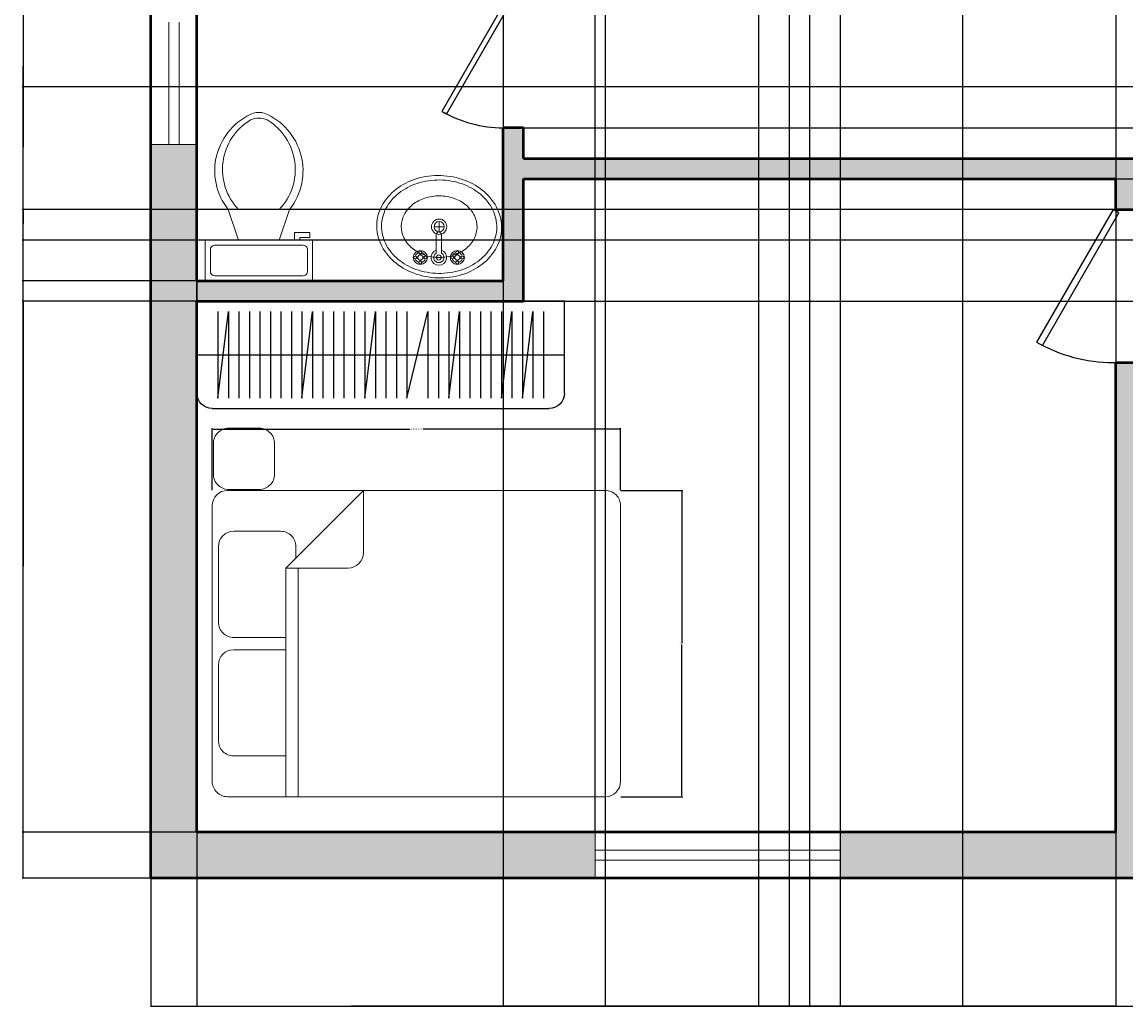
# Model space of a CAD drawing. Units: inches. Extents: x 3439 to 3988, y 1915 to 2284.
# Tile 1 of 7: x 3439 to 3656, y 1915 to 2108. Entities that reach past the tile are written whole.
import ezdxf

# ---------------------------------------------------------------- set-up
doc = ezdxf.new("R2010")
doc.units = ezdxf.units.IN
for name, color, linetype, lineweight in [('A-ANNO-DIMS', 2, 'Continuous', 18), ('A-DOOR', 3, 'Continuous', 25), ('A-FLOR-CASE', 8, 'Continuous', 25), ('A-FLOR-FIXT', 9, 'Continuous', 18), ('A-FURN', 9, 'Continuous', 18), ('A-GLAZ', 4, 'Continuous', 18), ('A-WALL', 7, 'Continuous', 50)]:
    doc.layers.add(name, color=color, linetype=linetype, lineweight=lineweight)
doc.layers.add('A-WALL-PATT', color=18, linetype='Continuous', lineweight=13, true_color=0x000000)
doc.styles.get("Standard").update_dxf_attribs({"font": 'arial.ttf'})
doc.dimstyles.get("Standard").update_dxf_attribs({"dimtxt": 0.18, "dimasz": 0.18, "dimexe": 0.18, "dimexo": 0.0625, "dimgap": 0.09, "dimtad": 0, "dimtih": 1, "dimtoh": 1, "dimdec": 4, "dimzin": 0, "dimdsep": 46, "dimtxsty": 'Standard', "dimcen": 0.09, "dimadec": 0, "dimazin": 0, "dimtfac": 1, "dimtdec": 4, "dimtofl": 0, "dimtmove": 0, "dimatfit": 3, "dimfxl": 1, "dimtolj": 1, "dimtzin": 0, "dimarcsym": 0})

# ---------------------------------------------------------------- blocks, each defined once
blk = doc.blocks.new('*U5')
for p, q in [((0, 0), (0, 6)), ((40, 0), (40, 6))]:
    blk.add_line(p, q)
blk.add_lwpolyline([(0, 0), (34.64, -20), (35.52, -18.48), (0.87, 1.52)], close=True)
blk.add_arc((0, 0), 40, 330, 0)
blk = doc.blocks.new('Bed - Queen')
for p, q in [((3, 0), (56.99999, 0)), ((10.99999, -1.2), (25.79998, -1.2)), ((34.19999, -1.2), (48.99999, -1.2)), ((0, -77.00003), (0, -3)), ((7.99999, -14.4), (7.99999, -4.2)), ((28.79998, -4.2), (28.79998, -14.4)), ((31.19999, -14.4), (31.19999, -4.2)), ((51.99999, -4.2), (51.99999, -13.4)), ((59.99999, -3), (59.99999, -77.00003)), ((0, -14.4), (44.8, -14.4)), ((59.99999, -29.6), (44.8, -14.4)), ((44.8, -14.4), (44.8, -26.6)), ((44.8, -16.8), (0, -16.8)), ((48.99999, -16.4), (46.79936, -16.4)), ((47.8, -29.6), (59.99999, -29.6)), ((56.99999, -80.00003), (3, -80.00003))]:
    blk.add_line(p, q)
for centre, start, end in [((3, -3), 90, 180), ((56.99999, -3), 0, 90), ((10.99999, -4.2), 90, 180), ((25.79998, -4.2), 0, 90), ((34.19999, -4.2), 90, 180), ((48.99999, -4.2), 0, 90), ((48.99999, -13.4), 270, 0), ((47.8, -26.6), 180, 270), ((3, -77.00003), 180, 270), ((56.99999, -77.00003), 270, 0)]:
    blk.add_arc(centre, 3, start, end)
blk = doc.blocks.new('Toilet - top')
for p, q in [((9.5, -6), (9.5, -2)), ((-10, -8.5), (-8, -8.5)), ((-10, -9.5), (-10, -8.5)), ((-8, -8.5), (-8, -8)), ((-7, -8), (-7, -9.5)), ((-4, -8), (-6, -14)), ((4, -8), (6, -14)), ((-7, -9.5), (-10, -9.5)), ((4, -14), (-4, -14))]:
    blk.add_line(p, q)
blk.add_lwpolyline([(10.5, -8), (10.5, 0), (-10.5, 0), (-10.5, -8)], close=True)
for points in [[(-9.5, -2), (-9.5, -6)], [(8.5, -1), (-8.5, -1)], [(-8.5, -7), (8.5, -7)]]:
    blk.add_lwpolyline(points)
for centre, radius, start, end in [((-8.62, -1.88), 0.884, 81.8699, 188.1301), ((8.62, -1.88), 0.884, 351.8699, 98.1301), ((-8.62, -6.12), 0.884, 171.8699, 278.1301), ((8.62, -6.12), 0.884, 261.8699, 8.1301), ((3.52, -21.58), 12.17, 141.4691, 247.9714), ((4.2, -21.82), 11.33, 136.3677, 238.9468), ((-3.52, -21.58), 12.17, 292.0284, 38.5307), ((-4.2, -21.82), 11.33, 301.053, 43.6321), ((0, -27.88), 4, 245.7318, 294.2682), ((0, -29), 4, 254.8605, 285.1395)]:
    blk.add_arc(centre, radius, start, end)
blk = doc.blocks.new('Sink - Oval top')
for p, q in [((-1, 0), (1, 0)), ((0, 1), (0, -1))]:
    blk.add_line(p, q)
for points in [[(-12.23, 0.39, 0.117634), (-11.46, -3.36, 0.104469), (-8.88, -6.8, 0.090016), (-5.08, -9.07, 0.08192), (-0.32, -10.02, 0.08192), (4.49, -9.38, 0.090016), (8.42, -7.36, 0.104469), (11.22, -4.09, 0.117634), (12.23, -0.39, 0.117634), (11.46, 3.36, 0.104469), (8.88, 6.8, 0.090016), (5.08, 9.07, 0.08192), (0.32, 10.02, 0.08192), (-4.49, 9.38, 0.090016), (-8.42, 7.36, 0.104469), (-11.22, 4.09, 0.117634)], [(-11.29, 0.16, 0.118622), (-10.52, -3.25, 0.104678), (-8.07, -6.36, 0.089562), (-4.54, -8.37, 0.081185), (-0.13, -9.15, 0.081185), (4.3, -8.49, 0.089562), (7.89, -6.58, 0.104678), (10.42, -3.55, 0.118622), (11.29, -0.16, 0.118622), (10.52, 3.25, 0.104678), (8.07, 6.36, 0.089562), (4.54, 8.37, 0.081185), (0.13, 9.15, 0.081185), (-4.3, 8.49, 0.089562), (-7.89, 6.58, 0.104678), (-10.42, 3.55, 0.118622)], [(-7.42, 0.08, 0.118283), (-6.91, -2.17, 0.104607), (-5.29, -4.21, 0.089718), (-2.97, -5.53, 0.081436), (-0.07, -6.04, 0.081436), (2.84, -5.59, 0.089718), (5.2, -4.33, 0.104607), (6.86, -2.32, 0.118283), (7.42, -0.08, 0.118283), (6.91, 2.17, 0.104607), (5.29, 4.21, 0.089718), (2.97, 5.53, 0.081436), (0.07, 6.04, 0.081436), (-2.84, 5.59, 0.089718), (-5.2, 4.33, 0.104607), (-6.86, 2.32, 0.118283)]]:
    blk.add_lwpolyline(points, format="xyb", close=True)
for radius in [1.5, 1]:
    blk.add_circle((0, 0), radius)
blk = doc.blocks.new('Faucet - Bathroom top')
for p, q in [((-4.107, 0.125), (-4.375, 0.125)), ((-3.75, 0.4788), (-3.75, 0.75)), ((-3.5, 0.482), (-3.5, 0.75)), ((-3.1461, 0.125), (-2.875, 0.125)), ((3.143, 0.125), (2.875, 0.125)), ((3.5, 0.4788), (3.5, 0.75)), ((3.75, 0.482), (3.75, 0.75)), ((4.1039, 0.125), (4.375, 0.125)), ((-4.1039, -0.125), (-4.375, -0.125)), ((-3.75, -0.4821), (-3.75, -0.75)), ((-3.5, -0.4789), (-3.5, -0.75)), ((-3.143, -0.125), (-2.875, -0.125)), ((-0.5, -0.8639), (-0.5, -4.5)), ((0.5, -4.5), (0.5, -0.8631)), ((3.1461, -0.125), (2.875, -0.125)), ((3.5, -0.4821), (3.5, -0.75)), ((3.75, -0.4789), (3.75, -0.75)), ((4.107, -0.125), (4.375, -0.125))]:
    blk.add_line(p, q)
for centre, radius in [((-3.625, 0), 1.375), ((-4.625, 0), 0.2795), ((-3.625, 0), 0.5), ((-3.625, 1), 0.2795), ((-2.625, 0), 0.2795), ((0, 0), 0.5), ((3.625, 0), 1.375), ((2.625, 0), 0.2795), ((3.625, 0), 0.5), ((3.625, 1), 0.2795), ((4.625, 0), 0.2795), ((-3.625, -1), 0.2795), ((3.625, -1), 0.2795)]:
    blk.add_circle(centre, radius)
for centre, radius, start, end in [((-3.625, 0), 1, 105.2407, 164.2093), ((-3.625, 0), 1, 16.44125, 74.07887), ((0, 0), 1.5, 289.6514, 250.3603), ((0, 0), 1, 300.3431, 239.7554), ((3.625, 0), 1, 106.12, 164.0884), ((3.625, 0), 1, 16.23422, 73.90469), ((-3.625, 0), 1, 196.2342, 253.9047), ((-3.625, 0), 1, 286.12, 344.0884), ((3.625, 0), 1, 196.4413, 254.0789), ((3.625, 0), 1, 285.2407, 344.2093), ((0, -4.5), 0.5, 180, 0)]:
    blk.add_arc(centre, radius, start, end)
blk = doc.blocks.new('WINDOW-GLASS-48IN')
for p, q in [((0, 2), (48, 2)), ((0, 0), (48, 0))]:
    blk.add_line(p, q)
blk = doc.blocks.new('WINDOW-GLASS-24IN')
for p, q in [((0, 2), (24, 2)), ((0, 0), (24, 0))]:
    blk.add_line(p, q)
blk = doc.blocks.new('WARDROBE-72IN')
for p, q in [((3, 21), (69, 21)), ((0, 0), (0, 18)), ((4.11, 2), (4.11, 19)), ((4.11, 19), (6.17, 2)), ((6.17, 2), (6.17, 19)), ((8.23, 2), (8.23, 19)), ((10.28, 2), (10.28, 19)), ((12.34, 2), (12.34, 19)), ((14.4, 2), (14.4, 19)), ((16.45, 2), (16.45, 19)), ((18.51, 2), (18.51, 19)), ((20.57, 2), (20.57, 19)), ((20.57, 19), (22.62, 2)), ((22.62, 2), (22.62, 19)), ((24.68, 2), (24.68, 19)), ((26.74, 2), (26.74, 19)), ((28.79, 2), (28.79, 19)), ((30.85, 2), (30.85, 19)), ((32.91, 2), (32.91, 19)), ((32.91, 19), (34.97, 2)), ((34.97, 2), (34.97, 19)), ((37.02, 2), (37.02, 19)), ((39.08, 2), (39.08, 19)), ((41.14, 2), (41.14, 19)), ((41.14, 19), (45.25, 2)), ((45.25, 2), (45.25, 19)), ((47.31, 2), (47.31, 19)), ((49.36, 2), (49.36, 19)), ((49.36, 19), (51.42, 2)), ((51.42, 2), (51.42, 19)), ((53.48, 2), (53.48, 19)), ((55.53, 2), (55.53, 19)), ((57.59, 2), (57.59, 19)), ((59.65, 2), (59.65, 19)), ((59.65, 19), (61.7, 2)), ((61.7, 2), (61.7, 19)), ((63.76, 2), (63.76, 19)), ((63.76, 19), (65.82, 2)), ((65.82, 2), (65.82, 19)), ((67.87, 2), (67.87, 19)), ((72, 18), (72, 0)), ((0, 10.5), (72, 10.5)), ((72, 0), (0, 0))]:
    blk.add_line(p, q)
for centre, start, end in [((3, 18), 90, 180), ((69, 18), 0, 90)]:
    blk.add_arc(centre, 3, start, end)
blk = doc.blocks.new('NIGHTSTAND-12IN-RADIUS')
blk.add_lwpolyline([(3, 0), (9, 0, 0.414214), (12, 3), (12, 9, 0.414214), (9, 12), (3, 12, 0.414214), (0, 9), (0, 3, 0.414214)], format="xyb", close=True)
blk = doc.blocks.new('*D23')
at = {"layer": 'A-ANNO-DIMS', "color": 0, "lineweight": -2, "transparency": 16777216}
for p, q in [((3476.58, 2016.37), (3476.58, 2028.49)), ((3556.58, 2016.37), (3556.58, 2028.49)), ((3476.76, 2028.31), (3515.28, 2028.31)), ((3556.4, 2028.31), (3517.89, 2028.31))]:
    blk.add_line(p, q, dxfattribs=at)
at = {"layer": 'A-ANNO-DIMS', "color": 0, "transparency": 16777216}
for points in [[(3476.76, 2028.34), (3476.76, 2028.28), (3476.58, 2028.31)], [(3556.4, 2028.34), (3556.4, 2028.28), (3556.58, 2028.31)]]:
    blk.add_solid(points, dxfattribs=at)
at = {"layer": 'Defpoints', "color": 0, "transparency": 16777216}
for p in [(3476.58, 2028.31), (3476.58, 2016.31), (3556.58, 2016.31)]:
    blk.add_point(p, dxfattribs=at)
at = {"layer": 'A-ANNO-DIMS', "color": 0, "transparency": 16777216, "insert": (3516.58, 2028.31), "char_height": 0.18, "attachment_point": 5}
blk.add_mtext('\\A1;QUEEN BED 80 TYP.', dxfattribs=at)
blk = doc.blocks.new('*D24')
at = {"layer": 'A-ANNO-DIMS', "color": 0, "lineweight": -2, "transparency": 16777216}
for p, q in [((3556.65, 2016.31), (3568.76, 2016.31)), ((3568.58, 2016.13), (3568.58, 1986.49)), ((3568.58, 1956.49), (3568.58, 1986.13)), ((3556.65, 1956.31), (3568.76, 1956.31))]:
    blk.add_line(p, q, dxfattribs=at)
at = {"layer": 'A-ANNO-DIMS', "color": 0, "transparency": 16777216}
for points in [[(3568.55, 2016.13), (3568.61, 2016.13), (3568.58, 2016.31)], [(3568.55, 1956.49), (3568.61, 1956.49), (3568.58, 1956.31)]]:
    blk.add_solid(points, dxfattribs=at)
at = {"layer": 'Defpoints', "color": 0, "transparency": 16777216}
for p in [(3556.58, 2016.31), (3568.58, 2016.31), (3556.58, 1956.31)]:
    blk.add_point(p, dxfattribs=at)
at = {"layer": 'A-ANNO-DIMS', "color": 0, "transparency": 16777216, "insert": (3568.58, 1986.31), "char_height": 0.18, "attachment_point": 5}
blk.add_mtext('\\A1;60 TYP.', dxfattribs=at)
blk = doc.blocks.new('*D45')
at = {"layer": 'A-ANNO-DIMS', "color": 0, "lineweight": -2, "transparency": 16777216}
for p, q in [((3464.58, 1940.3), (3464.58, 1915.13)), ((3962.58, 1940.3), (3962.58, 1915.13)), ((3464.76, 1915.31), (3713.29, 1915.31)), ((3962.4, 1915.31), (3713.87, 1915.31))]:
    blk.add_line(p, q, dxfattribs=at)
at = {"layer": 'A-ANNO-DIMS', "color": 0, "transparency": 16777216}
for points in [[(3464.76, 1915.34), (3464.76, 1915.28), (3464.58, 1915.31)], [(3962.4, 1915.34), (3962.4, 1915.28), (3962.58, 1915.31)]]:
    blk.add_solid(points, dxfattribs=at)
at = {"layer": 'Defpoints', "color": 0, "transparency": 16777216}
for p in [(3464.58, 1940.36), (3962.58, 1940.36), (3962.58, 1915.31)]:
    blk.add_point(p, dxfattribs=at)
at = {"layer": 'A-ANNO-DIMS', "color": 0, "transparency": 16777216, "insert": (3713.58, 1915.31), "char_height": 0.18, "attachment_point": 5}
blk.add_mtext('\\A1;498', dxfattribs=at)
blk = doc.blocks.new('*D46')
at = {"layer": 'A-ANNO-DIMS', "color": 0, "lineweight": -2, "transparency": 16777216}
for p, q in [((3464.52, 2258.36), (3439.35, 2258.36)), ((3439.53, 2258.18), (3439.53, 2099.54)), ((3439.53, 1940.54), (3439.53, 2099.18)), ((3464.52, 1940.36), (3439.35, 1940.36))]:
    blk.add_line(p, q, dxfattribs=at)
at = {"layer": 'A-ANNO-DIMS', "color": 0, "transparency": 16777216}
for points in [[(3439.5, 2258.18), (3439.56, 2258.18), (3439.53, 2258.36)], [(3439.5, 1940.54), (3439.56, 1940.54), (3439.53, 1940.36)]]:
    blk.add_solid(points, dxfattribs=at)
at = {"layer": 'Defpoints', "color": 0, "transparency": 16777216}
for p in [(3439.53, 2258.36), (3464.58, 2258.36), (3464.58, 1940.36)]:
    blk.add_point(p, dxfattribs=at)
at = {"layer": 'A-ANNO-DIMS', "color": 0, "transparency": 16777216, "insert": (3439.53, 2099.36), "char_height": 0.18, "attachment_point": 5}
blk.add_mtext('\\A1;318', dxfattribs=at)
blk = doc.blocks.new('*D47')
at = {"layer": 'A-ANNO-DIMS', "color": 0, "lineweight": -2, "transparency": 16777216}
for p, q in [((3473.58, 2249.3), (3473.58, 1915.13)), ((3589.58, 2249.3), (3589.58, 1915.13)), ((3473.76, 1915.31), (3531.3, 1915.31)), ((3589.4, 1915.31), (3531.86, 1915.31))]:
    blk.add_line(p, q, dxfattribs=at)
at = {"layer": 'A-ANNO-DIMS', "color": 0, "transparency": 16777216}
for points in [[(3473.76, 1915.34), (3473.76, 1915.28), (3473.58, 1915.31)], [(3589.4, 1915.34), (3589.4, 1915.28), (3589.58, 1915.31)]]:
    blk.add_solid(points, dxfattribs=at)
at = {"layer": 'Defpoints', "color": 0, "transparency": 16777216}
for p in [(3473.58, 2249.36), (3589.58, 2249.36), (3589.58, 1915.31)]:
    blk.add_point(p, dxfattribs=at)
at = {"layer": 'A-ANNO-DIMS', "color": 0, "transparency": 16777216, "insert": (3531.58, 1915.31), "char_height": 0.18, "attachment_point": 5}
blk.add_mtext('\\A1;116', dxfattribs=at)
blk = doc.blocks.new('*D48')
at = {"layer": 'A-ANNO-DIMS', "color": 0, "lineweight": -2, "transparency": 16777216}
for p, q in [((3593.58, 2249.3), (3593.58, 1915.13)), ((3653.58, 2249.3), (3653.58, 1915.13)), ((3593.76, 1915.31), (3623.36, 1915.31)), ((3653.4, 1915.31), (3623.8, 1915.31))]:
    blk.add_line(p, q, dxfattribs=at)
at = {"layer": 'A-ANNO-DIMS', "color": 0, "transparency": 16777216}
for points in [[(3593.76, 1915.34), (3593.76, 1915.28), (3593.58, 1915.31)], [(3653.4, 1915.34), (3653.4, 1915.28), (3653.58, 1915.31)]]:
    blk.add_solid(points, dxfattribs=at)
at = {"layer": 'Defpoints', "color": 0, "transparency": 16777216}
for p in [(3593.58, 2249.36), (3653.58, 2249.36), (3653.58, 1915.31)]:
    blk.add_point(p, dxfattribs=at)
at = {"layer": 'A-ANNO-DIMS', "color": 0, "transparency": 16777216, "insert": (3623.58, 1915.31), "char_height": 0.18, "attachment_point": 5}
blk.add_mtext('\\A1;60', dxfattribs=at)
blk = doc.blocks.new('*D52')
at = {"layer": 'A-ANNO-DIMS', "color": 0, "lineweight": -2, "transparency": 16777216}
for p, q in [((3473.58, 1949.3), (3473.58, 1915.13)), ((3653.58, 1949.3), (3653.58, 1915.13)), ((3473.76, 1915.31), (3563.3, 1915.31)), ((3653.4, 1915.31), (3563.86, 1915.31))]:
    blk.add_line(p, q, dxfattribs=at)
at = {"layer": 'A-ANNO-DIMS', "color": 0, "transparency": 16777216}
for points in [[(3473.76, 1915.34), (3473.76, 1915.28), (3473.58, 1915.31)], [(3653.4, 1915.34), (3653.4, 1915.28), (3653.58, 1915.31)]]:
    blk.add_solid(points, dxfattribs=at)
at = {"layer": 'Defpoints', "color": 0, "transparency": 16777216}
for p in [(3473.58, 1949.36), (3653.58, 1949.36), (3653.58, 1915.31)]:
    blk.add_point(p, dxfattribs=at)
at = {"layer": 'A-ANNO-DIMS', "color": 0, "transparency": 16777216, "insert": (3563.58, 1915.31), "char_height": 0.18, "attachment_point": 5}
blk.add_mtext('\\A1;180', dxfattribs=at)
blk = doc.blocks.new('*D56')
at = {"layer": 'A-ANNO-DIMS', "color": 0, "lineweight": -2, "transparency": 16777216}
for p, q in [((3473.52, 2129.36), (3439.35, 2129.36)), ((3439.53, 2129.18), (3439.53, 2093.54)), ((3439.53, 2057.54), (3439.53, 2093.18)), ((3473.52, 2057.36), (3439.35, 2057.36))]:
    blk.add_line(p, q, dxfattribs=at)
at = {"layer": 'A-ANNO-DIMS', "color": 0, "transparency": 16777216}
for points in [[(3439.5, 2129.18), (3439.56, 2129.18), (3439.53, 2129.36)], [(3439.5, 2057.54), (3439.56, 2057.54), (3439.53, 2057.36)]]:
    blk.add_solid(points, dxfattribs=at)
at = {"layer": 'Defpoints', "color": 0, "transparency": 16777216}
for p in [(3439.53, 2129.36), (3473.58, 2129.36), (3473.58, 2057.36)]:
    blk.add_point(p, dxfattribs=at)
at = {"layer": 'A-ANNO-DIMS', "color": 0, "transparency": 16777216, "insert": (3439.53, 2093.36), "char_height": 0.18, "attachment_point": 5}
blk.add_mtext('\\A1;72', dxfattribs=at)
blk = doc.blocks.new('*D57')
at = {"layer": 'A-ANNO-DIMS', "color": 0, "lineweight": -2, "transparency": 16777216}
for p, q in [((3473.52, 2053.36), (3439.35, 2053.36)), ((3439.53, 2053.18), (3439.53, 2001.54)), ((3439.53, 1949.54), (3439.53, 2001.18)), ((3473.52, 1949.36), (3439.35, 1949.36))]:
    blk.add_line(p, q, dxfattribs=at)
at = {"layer": 'A-ANNO-DIMS', "color": 0, "transparency": 16777216}
for points in [[(3439.5, 2053.18), (3439.56, 2053.18), (3439.53, 2053.36)], [(3439.5, 1949.54), (3439.56, 1949.54), (3439.53, 1949.36)]]:
    blk.add_solid(points, dxfattribs=at)
at = {"layer": 'Defpoints', "color": 0, "transparency": 16777216}
for p in [(3439.53, 2053.36), (3473.58, 2053.36), (3473.58, 1949.36)]:
    blk.add_point(p, dxfattribs=at)
at = {"layer": 'A-ANNO-DIMS', "color": 0, "transparency": 16777216, "insert": (3439.53, 2001.36), "char_height": 0.18, "attachment_point": 5}
blk.add_mtext('\\A1;104', dxfattribs=at)
blk = doc.blocks.new('*D61')
at = {"layer": 'A-ANNO-DIMS', "color": 0, "lineweight": -2, "transparency": 16777216}
for p, q in [((3473.58, 2129.3), (3473.58, 1915.13)), ((3533.58, 2129.3), (3533.58, 1915.13)), ((3473.76, 1915.31), (3503.36, 1915.31)), ((3533.4, 1915.31), (3503.8, 1915.31))]:
    blk.add_line(p, q, dxfattribs=at)
at = {"layer": 'A-ANNO-DIMS', "color": 0, "transparency": 16777216}
for points in [[(3473.76, 1915.34), (3473.76, 1915.28), (3473.58, 1915.31)], [(3533.4, 1915.34), (3533.4, 1915.28), (3533.58, 1915.31)]]:
    blk.add_solid(points, dxfattribs=at)
at = {"layer": 'Defpoints', "color": 0, "transparency": 16777216}
for p in [(3473.58, 2129.36), (3533.58, 2129.36), (3533.58, 1915.31)]:
    blk.add_point(p, dxfattribs=at)
at = {"layer": 'A-ANNO-DIMS', "color": 0, "transparency": 16777216, "insert": (3503.58, 1915.31), "char_height": 0.18, "attachment_point": 5}
blk.add_mtext('\\A1;60', dxfattribs=at)
blk = doc.blocks.new('*D62')
at = {"layer": 'A-ANNO-DIMS', "color": 0, "lineweight": -2, "transparency": 16777216}
for p, q in [((3537.64, 2077.36), (3987.81, 2077.36)), ((3987.63, 2077.18), (3987.63, 2065.54)), ((3987.63, 2053.54), (3987.63, 2065.18)), ((3537.64, 2053.36), (3987.81, 2053.36))]:
    blk.add_line(p, q, dxfattribs=at)
at = {"layer": 'A-ANNO-DIMS', "color": 0, "transparency": 16777216}
for points in [[(3987.6, 2077.18), (3987.66, 2077.18), (3987.63, 2077.36)], [(3987.6, 2053.54), (3987.66, 2053.54), (3987.63, 2053.36)]]:
    blk.add_solid(points, dxfattribs=at)
at = {"layer": 'Defpoints', "color": 0, "transparency": 16777216}
for p in [(3537.58, 2077.36), (3987.63, 2077.36), (3537.58, 2053.36)]:
    blk.add_point(p, dxfattribs=at)
at = {"layer": 'A-ANNO-DIMS', "color": 0, "transparency": 16777216, "insert": (3987.63, 2065.36), "char_height": 0.18, "attachment_point": 5}
blk.add_mtext('\\A1;24', dxfattribs=at)
blk = doc.blocks.new('*D72')
at = {"layer": 'A-ANNO-DIMS', "color": 0, "lineweight": -2, "transparency": 16777216}
for p, q in [((3473.58, 1949.42), (3473.58, 2284)), ((3473.76, 2283.82), (3512.21, 2283.82)), ((3551.44, 2283.82), (3512.99, 2283.82)), ((3551.62, 1949.42), (3551.62, 2284))]:
    blk.add_line(p, q, dxfattribs=at)
at = {"layer": 'A-ANNO-DIMS', "color": 0, "transparency": 16777216}
for points in [[(3473.76, 2283.85), (3473.76, 2283.79), (3473.58, 2283.82)], [(3551.44, 2283.85), (3551.44, 2283.79), (3551.62, 2283.82)]]:
    blk.add_solid(points, dxfattribs=at)
at = {"layer": 'Defpoints', "color": 0, "transparency": 16777216}
for p in [(3551.62, 2283.82), (3473.58, 1949.36), (3551.62, 1949.36)]:
    blk.add_point(p, dxfattribs=at)
at = {"layer": 'A-ANNO-DIMS', "color": 0, "transparency": 16777216, "insert": (3512.6, 2283.82), "char_height": 0.18, "attachment_point": 5}
blk.add_mtext('\\A1;78.04', dxfattribs=at)
blk = doc.blocks.new('*D78')
at = {"layer": 'A-ANNO-DIMS', "color": 0, "lineweight": -2, "transparency": 16777216}
for p, q in [((3553.58, 2129.3), (3553.58, 1915.13)), ((3583.58, 2129.3), (3583.58, 1915.13)), ((3553.76, 1915.31), (3568.36, 1915.31)), ((3583.4, 1915.31), (3568.8, 1915.31))]:
    blk.add_line(p, q, dxfattribs=at)
at = {"layer": 'A-ANNO-DIMS', "color": 0, "transparency": 16777216}
for points in [[(3553.76, 1915.34), (3553.76, 1915.28), (3553.58, 1915.31)], [(3583.4, 1915.34), (3583.4, 1915.28), (3583.58, 1915.31)]]:
    blk.add_solid(points, dxfattribs=at)
at = {"layer": 'Defpoints', "color": 0, "transparency": 16777216}
for p in [(3553.58, 2129.36), (3583.58, 2129.36), (3583.58, 1915.31)]:
    blk.add_point(p, dxfattribs=at)
at = {"layer": 'A-ANNO-DIMS', "color": 0, "transparency": 16777216, "insert": (3568.58, 1915.31), "char_height": 0.18, "attachment_point": 5}
blk.add_mtext('\\A1;30', dxfattribs=at)
blk = doc.blocks.new('*D80')
at = {"layer": 'A-ANNO-DIMS', "color": 0, "lineweight": -2, "transparency": 16777216}
for p, q in [((3599.58, 2141.3), (3599.58, 1915.13)), ((3623.58, 2141.3), (3623.58, 1915.13)), ((3599.76, 1915.31), (3611.36, 1915.31)), ((3623.4, 1915.31), (3611.8, 1915.31))]:
    blk.add_line(p, q, dxfattribs=at)
at = {"layer": 'A-ANNO-DIMS', "color": 0, "transparency": 16777216}
for points in [[(3599.76, 1915.34), (3599.76, 1915.28), (3599.58, 1915.31)], [(3623.4, 1915.34), (3623.4, 1915.28), (3623.58, 1915.31)]]:
    blk.add_solid(points, dxfattribs=at)
at = {"layer": 'Defpoints', "color": 0, "transparency": 16777216}
for p in [(3599.58, 2141.36), (3623.58, 2141.36), (3623.58, 1915.31)]:
    blk.add_point(p, dxfattribs=at)
at = {"layer": 'A-ANNO-DIMS', "color": 0, "transparency": 16777216, "insert": (3611.58, 1915.31), "char_height": 0.18, "attachment_point": 5}
blk.add_mtext('\\A1;24', dxfattribs=at)
blk = doc.blocks.new('*D83')
at = {"layer": 'A-ANNO-DIMS', "color": 0, "lineweight": -2, "transparency": 16777216}
for p, q in [((3537.64, 2111.36), (3987.81, 2111.36)), ((3987.63, 2111.18), (3987.63, 2099.54)), ((3987.63, 2087.54), (3987.63, 2099.18)), ((3537.64, 2087.36), (3987.81, 2087.36))]:
    blk.add_line(p, q, dxfattribs=at)
at = {"layer": 'A-ANNO-DIMS', "color": 0, "transparency": 16777216}
for points in [[(3987.6, 2111.18), (3987.66, 2111.18), (3987.63, 2111.36)], [(3987.6, 2087.54), (3987.66, 2087.54), (3987.63, 2087.36)]]:
    blk.add_solid(points, dxfattribs=at)
at = {"layer": 'Defpoints', "color": 0, "transparency": 16777216}
for p in [(3537.58, 2111.36), (3987.63, 2111.36), (3537.58, 2087.36)]:
    blk.add_point(p, dxfattribs=at)
at = {"layer": 'A-ANNO-DIMS', "color": 0, "transparency": 16777216, "insert": (3987.63, 2099.36), "char_height": 0.18, "attachment_point": 5}
blk.add_mtext('\\A1;24', dxfattribs=at)
blk = doc.blocks.new('*D88')
at = {"layer": 'A-ANNO-DIMS', "color": 0, "lineweight": -2, "transparency": 16777216}
for p, q in [((3653.64, 2077.36), (3987.81, 2077.36)), ((3987.63, 2077.18), (3987.63, 2074.54)), ((3987.63, 2071.54), (3987.63, 2074.18)), ((3653.64, 2071.36), (3987.81, 2071.36))]:
    blk.add_line(p, q, dxfattribs=at)
at = {"layer": 'A-ANNO-DIMS', "color": 0, "transparency": 16777216}
for points in [[(3987.6, 2077.18), (3987.66, 2077.18), (3987.63, 2077.36)], [(3987.6, 2071.54), (3987.66, 2071.54), (3987.63, 2071.36)]]:
    blk.add_solid(points, dxfattribs=at)
at = {"layer": 'Defpoints', "color": 0, "transparency": 16777216}
for p in [(3653.58, 2077.36), (3987.63, 2077.36), (3653.58, 2071.36)]:
    blk.add_point(p, dxfattribs=at)
at = {"layer": 'A-ANNO-DIMS', "color": 0, "transparency": 16777216, "insert": (3987.63, 2074.36), "char_height": 0.18, "attachment_point": 5}
blk.add_mtext('\\A1;6', dxfattribs=at)
blk = doc.blocks.new('*D90')
at = {"layer": 'A-ANNO-DIMS', "color": 0, "lineweight": -2, "transparency": 16777216}
for p, q in [((3889.52, 2071.36), (3439.35, 2071.36)), ((3439.53, 2071.18), (3439.53, 2068.54)), ((3439.53, 2065.54), (3439.53, 2068.18)), ((3889.52, 2065.36), (3439.35, 2065.36))]:
    blk.add_line(p, q, dxfattribs=at)
at = {"layer": 'A-ANNO-DIMS', "color": 0, "transparency": 16777216}
for points in [[(3439.5, 2071.18), (3439.56, 2071.18), (3439.53, 2071.36)], [(3439.5, 2065.54), (3439.56, 2065.54), (3439.53, 2065.36)]]:
    blk.add_solid(points, dxfattribs=at)
at = {"layer": 'Defpoints', "color": 0, "transparency": 16777216}
for p in [(3439.53, 2071.36), (3889.58, 2071.36), (3889.58, 2065.36)]:
    blk.add_point(p, dxfattribs=at)
at = {"layer": 'A-ANNO-DIMS', "color": 0, "transparency": 16777216, "insert": (3439.53, 2068.36), "char_height": 0.18, "attachment_point": 5}
blk.add_mtext('\\A1;6', dxfattribs=at)
blk = doc.blocks.new('*D91')
at = {"layer": 'A-ANNO-DIMS', "color": 0, "lineweight": -2, "transparency": 16777216}
for p, q in [((3889.52, 2095.36), (3439.35, 2095.36)), ((3439.53, 2095.18), (3439.53, 2083.54)), ((3439.53, 2071.54), (3439.53, 2083.18)), ((3889.52, 2071.36), (3439.35, 2071.36))]:
    blk.add_line(p, q, dxfattribs=at)
at = {"layer": 'A-ANNO-DIMS', "color": 0, "transparency": 16777216}
for points in [[(3439.5, 2095.18), (3439.56, 2095.18), (3439.53, 2095.36)], [(3439.5, 2071.54), (3439.56, 2071.54), (3439.53, 2071.36)]]:
    blk.add_solid(points, dxfattribs=at)
at = {"layer": 'Defpoints', "color": 0, "transparency": 16777216}
for p in [(3439.53, 2095.36), (3889.58, 2095.36), (3889.58, 2071.36)]:
    blk.add_point(p, dxfattribs=at)
at = {"layer": 'A-ANNO-DIMS', "color": 0, "transparency": 16777216, "insert": (3439.53, 2083.36), "char_height": 0.18, "attachment_point": 5}
blk.add_mtext('\\A1;24', dxfattribs=at)

msp = doc.modelspace()

# ---------------------------------------------------------------- hatches: boundary and pattern name
at = {"layer": 'A-WALL-PATT'}
h = msp.add_hatch(color=256, dxfattribs=at)
h.dxf.hatch_style = 1
h.paths.add_polyline_path([(3551.6168, 1949.3617), (3473.5815, 1949.3617), (3473.5815, 2053.3617), (3537.5815, 2053.3617), (3537.5815, 2077.3617), (3653.5815, 2077.3617), (3653.5815, 2071.3617), (3657.5815, 2071.3617), (3657.5815, 2081.3617), (3537.5815, 2081.3617), (3537.5815, 2087.3617), (3533.5815, 2087.3617), (3533.5815, 2057.3617), (3473.5815, 2057.3617), (3473.5815, 2084.0664), (3464.5815, 2084.0664), (3464.5815, 1940.3617), (3551.6168, 1940.3617)])
h = msp.add_hatch(color=256, dxfattribs=at)
h.dxf.hatch_style = 1
h.paths.add_polyline_path([(3664.1118, 1949.3617), (3657.5815, 1949.3617), (3657.5815, 2041.3617), (3653.5815, 2041.3617), (3653.5815, 1949.3617), (3599.6168, 1949.3617), (3599.6168, 1940.3617), (3664.1118, 1940.3617)])

# ---------------------------------------------------------------- linework, layer by layer
at = {"layer": 'A-GLAZ'}
for points in [[(3473.5815, 2084.0664), (3464.5815, 2084.0664)], [(3551.6168, 1940.3617), (3551.6168, 1949.3617)], [(3599.6168, 1949.3617), (3599.6168, 1940.3617)]]:
    msp.add_lwpolyline(points, dxfattribs=at)
at = {"layer": 'A-WALL'}
for p, q in [((3473.5815, 2057.3617), (3473.5815, 2129.3617)), ((3533.5815, 2057.3617), (3533.5815, 2087.3617)), ((3537.5815, 2087.3617), (3533.5815, 2087.3617)), ((3537.5815, 2081.3617), (3537.5815, 2087.3617)), ((3537.5815, 2081.3617), (3657.5815, 2081.3617)), ((3537.5815, 2057.3617), (3537.5815, 2077.3617)), ((3537.5815, 2053.3617), (3537.5815, 2077.3617)), ((3537.5815, 2077.3617), (3653.5815, 2077.3617)), ((3653.5815, 2071.3617), (3653.5815, 2077.3617)), ((3653.5815, 2071.3617), (3657.5815, 2071.3617)), ((3473.5815, 2057.3617), (3533.5815, 2057.3617)), ((3473.5815, 1949.3617), (3473.5815, 2053.3617)), ((3473.5815, 2053.3617), (3537.5815, 2053.3617)), ((3653.5815, 1949.3617), (3653.5815, 2041.3617)), ((3653.5815, 2041.3617), (3657.5815, 2041.3617)), ((3593.5815, 1949.3617), (3473.5815, 1949.3617)), ((3653.5815, 1949.3617), (3593.5815, 1949.3617))]:
    msp.add_line(p, q, dxfattribs=at)
msp.add_lwpolyline([(3719.5815, 1940.3617), (3464.5815, 1940.3617), (3464.5815, 2258.3617), (3803.9319, 2258.3617)], dxfattribs=at)

# ---------------------------------------------------------------- block references
at = {"layer": 'A-DOOR', "rotation": 270}
for p, xscale, yscale, zscale in [((3533.5815, 2111.3617), 0.6000000000000001, 0.6000000000000001, 0.6000000000000001), ((3653.0815, 2071.3617), 0.75, 0.75, 0.75)]:
    msp.add_blockref('*U5', p, dxfattribs=dict(at, xscale=xscale, yscale=yscale, zscale=zscale))
at = {"layer": 'A-FLOR-CASE', "extrusion": (0, 0, -1), "zscale": -1, "rotation": 180}
msp.add_blockref('WARDROBE-72IN', (-3473.5815, 2053.3617), dxfattribs=at)
at = {"layer": 'A-FLOR-FIXT', "rotation": 180}
for name, p in [('Toilet - top', (3485.7189, 2057.3617)), ('Sink - Oval top', (3521.0386, 2067.9813)), ('Faucet - Bathroom top', (3520.9711, 2061.9445))]:
    msp.add_blockref(name, p, dxfattribs=at)
at = {"layer": 'A-FURN'}
msp.add_blockref('NIGHTSTAND-12IN-RADIUS', (3476.798, 2016.5049), dxfattribs=at)
at = {"layer": 'A-FURN', "rotation": 89.99999999999999}
msp.add_blockref('Bed - Queen', (3476.5834, 1956.3099), dxfattribs=at)
at = {"layer": 'A-GLAZ', "rotation": 90.0000000000043}
msp.add_blockref('WINDOW-GLASS-24IN', (3470.0815, 2084.0664), dxfattribs=at)
at = {"layer": 'A-GLAZ'}
msp.add_blockref('WINDOW-GLASS-48IN', (3551.6168, 1943.8617), dxfattribs=at)

# ---------------------------------------------------------------- dimensions: what is measured, and where the dimension line sits
at = {"layer": 'A-ANNO-DIMS'}
for base, p1, p2, override, picture, middle in [((3551.6168, 2283.8228), (3473.5815, 1949.3617), (3551.6168, 1949.3617), {"dimdec": 2, "dimlfac": 1, "dimrnd": 0, "dimzin": 0, "dimdsep": 46, "dimlunit": 2}, '*D72', (3512.5992, 2283.8228)), ((3589.5815, 1915.3117), (3473.5815, 2249.3617), (3589.5815, 2249.3617), {"dimdec": 0, "dimlfac": 1, "dimrnd": 0, "dimzin": 0, "dimdsep": 46, "dimlunit": 2}, '*D47', (3531.5815, 1915.3117)), ((3653.5815, 1915.3117), (3593.5815, 2249.3617), (3653.5815, 2249.3617), {"dimdec": 0, "dimlfac": 1, "dimrnd": 0, "dimzin": 0, "dimdsep": 46, "dimlunit": 2}, '*D48', (3623.5815, 1915.3117)), ((3623.5815, 1915.3117), (3599.5815, 2141.3617), (3623.5815, 2141.3617), {"dimdec": 0, "dimlfac": 1, "dimrnd": 0, "dimzin": 0, "dimdsep": 46, "dimlunit": 2}, '*D80', (3611.5815, 1915.3117)), ((3533.5815, 1915.3117), (3473.5815, 2129.3617), (3533.5815, 2129.3617), {"dimdec": 0, "dimlfac": 1, "dimrnd": 0, "dimzin": 0, "dimdsep": 46, "dimlunit": 2}, '*D61', (3503.5815, 1915.3117)), ((3583.5815, 1915.3117), (3553.5815, 2129.3617), (3583.5815, 2129.3617), {"dimdec": 0, "dimlfac": 1, "dimrnd": 0, "dimzin": 0, "dimdsep": 46, "dimlunit": 2}, '*D78', (3568.5815, 1915.3117)), ((3653.5815, 1915.3117), (3473.5815, 1949.3617), (3653.5815, 1949.3617), {"dimdec": 0, "dimlfac": 1, "dimrnd": 0, "dimzin": 0, "dimdsep": 46, "dimlunit": 2}, '*D52', (3563.5815, 1915.3117)), ((3962.5815, 1915.3117), (3464.5815, 1940.3617), (3962.5815, 1940.3617), {"dimdec": 0, "dimlfac": 1, "dimrnd": 0, "dimzin": 0, "dimdsep": 46, "dimlunit": 2}, '*D45', (3713.5815, 1915.3117))]:
    dim = msp.add_linear_dim(base=base, p1=p1, p2=p2, dimstyle='Standard', override=override, dxfattribs=at)
    dim.commit()
    dim.dimension.update_dxf_attribs({"geometry": picture, "text_midpoint": middle})
for base, p1, p2, picture, middle in [((3439.5315, 2258.3617), (3464.5815, 1940.3617), (3464.5815, 2258.3617), '*D46', (3439.5315, 2099.3617)), ((3439.5315, 2129.3617), (3473.5815, 2057.3617), (3473.5815, 2129.3617), '*D56', (3439.5315, 2093.3617)), ((3987.6315, 2111.3617), (3537.5815, 2087.3617), (3537.5815, 2111.3617), '*D83', (3987.6315, 2099.3617)), ((3439.5315, 2095.3617), (3889.5815, 2071.3617), (3889.5815, 2095.3617), '*D91', (3439.5315, 2083.3617)), ((3987.6315, 2077.3617), (3537.5815, 2053.3617), (3537.5815, 2077.3617), '*D62', (3987.6315, 2065.3617)), ((3987.6315, 2077.3617), (3653.5815, 2071.3617), (3653.5815, 2077.3617), '*D88', (3987.6315, 2074.3617)), ((3439.5315, 2071.3617), (3889.5815, 2065.3617), (3889.5815, 2071.3617), '*D90', (3439.5315, 2068.3617)), ((3439.5315, 2053.3617), (3473.5815, 1949.3617), (3473.5815, 2053.3617), '*D57', (3439.5315, 2001.3617))]:
    dim = msp.add_linear_dim(base=base, p1=p1, p2=p2, angle=90, dimstyle='Standard', override={"dimdec": 0, "dimlfac": 1, "dimrnd": 0, "dimzin": 0, "dimdsep": 46, "dimlunit": 2}, dxfattribs=at)
    dim.commit()
    dim.dimension.update_dxf_attribs({"geometry": picture, "text_midpoint": middle})
for base, p1, p2, angle, text, picture, middle in [((3476.5834, 2028.3098), (3556.5835, 2016.3098), (3476.5834, 2016.3098), 180, 'QUEEN BED <> TYP.', '*D23', (3516.5834, 2028.3098)), ((3568.5835, 2016.3098), (3556.5835, 1956.3099), (3556.5835, 2016.3098), 90, '<> TYP.', '*D24', (3568.5835, 1986.3098))]:
    dim = msp.add_linear_dim(base=base, p1=p1, p2=p2, angle=angle, text=text, dimstyle='Standard', override={"dimdec": 0, "dimlfac": 1, "dimrnd": 0, "dimzin": 0, "dimdsep": 46, "dimlunit": 2}, dxfattribs=at)
    dim.commit()
    dim.dimension.update_dxf_attribs({"geometry": picture, "text_midpoint": middle})

doc.saveas('drawing.dxf')
